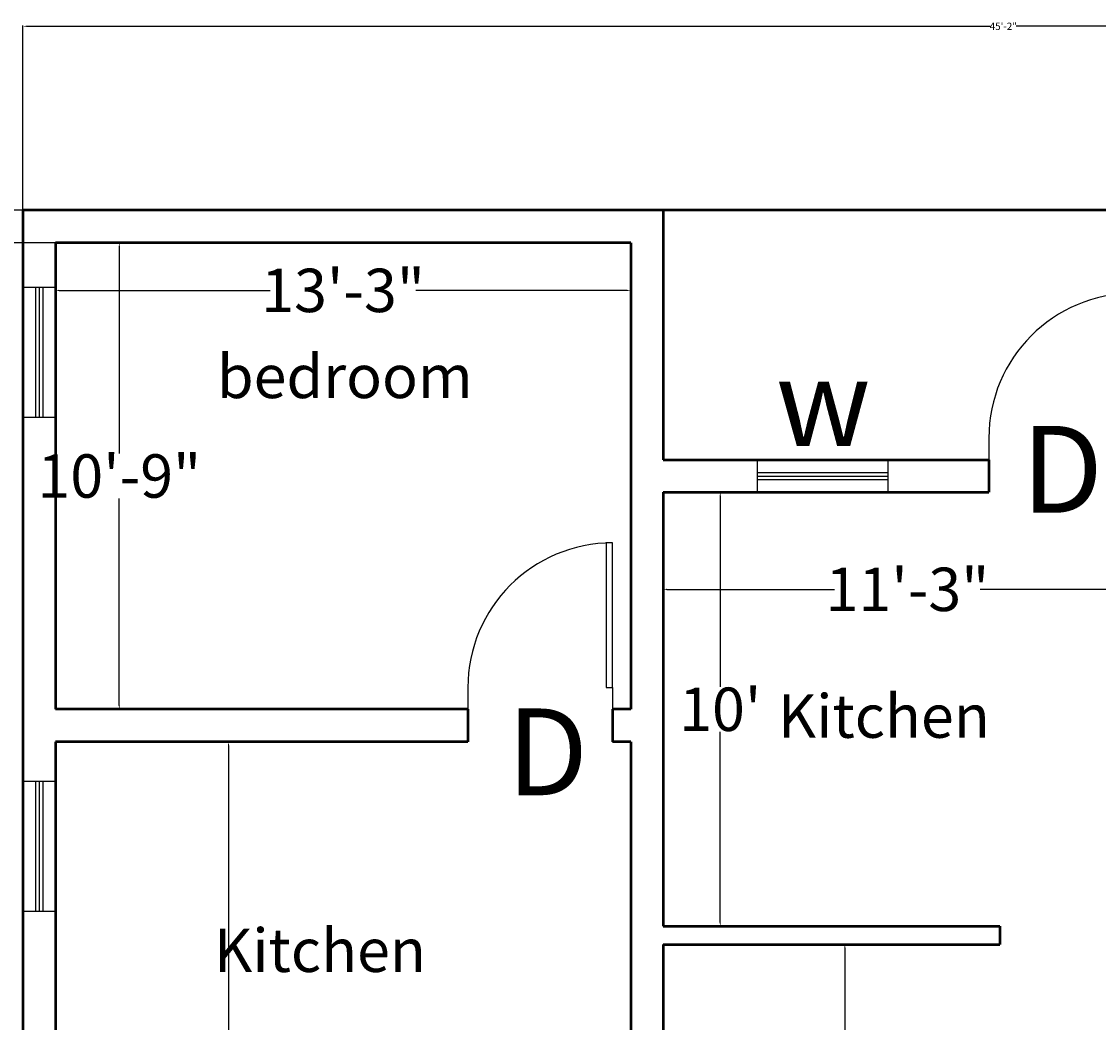
# Model space of a CAD drawing. Units: inches. Extents: x 409 to 7572, y 7 to 725.
# Tile 24 of 38: x 4326 to 4623, y 448 to 725. Entities that reach past the tile are written whole.
import ezdxf

# ---------------------------------------------------------------- set-up
doc = ezdxf.new("R2010")
doc.units = ezdxf.units.IN
doc.header["$MEASUREMENT"] = 0
for name, color, linetype, lineweight in [('A-ANNO-DIMS', 2, 'Continuous', 18), ('A-ANNO-SYMB', 3, 'Continuous', 25), ('A-AREA-IDEN', 7, 'Continuous', 25), ('A-DOOR', 3, 'Continuous', 25), ('A-GLAZ', 4, 'Continuous', 25), ('A-WALL', 7, 'Continuous', 50)]:
    doc.layers.add(name, color=color, linetype=linetype, lineweight=lineweight)
doc.styles.get("Standard").update_dxf_attribs({"font": 'arial.ttf'})
doc.dimstyles.get("Standard").update_dxf_attribs({"dimtxt": 2, "dimasz": 1, "dimexe": 0.18, "dimexo": 0.0625, "dimgap": 0.09, "dimtad": 0, "dimtih": 1, "dimtoh": 1, "dimdec": 0, "dimzin": 0, "dimdsep": 46, "dimlunit": 3, "dimtxsty": 'Standard', "dimcen": 0.09, "dimadec": 0, "dimazin": 0, "dimtfac": 1, "dimtdec": 0, "dimtofl": 0, "dimtmove": 0, "dimatfit": 3, "dimfxl": 1, "dimtolj": 1, "dimtzin": 0, "dimarcsym": 0})

# ---------------------------------------------------------------- blocks, each defined once
blk = doc.blocks.new('*U2')
for p, q in [((0, 0), (0, -6)), ((-40, 0), (-40, -6))]:
    blk.add_line(p, q)
blk.add_lwpolyline([(0, 0), (0, 40), (-1.75, 40), (-1.75, 0)], close=True)
blk.add_arc((0, 0), 40, 90, 180)
blk = doc.blocks.new('*D99')
at = {"layer": 'A-ANNO-DIMS', "color": 0, "lineweight": -2, "transparency": 16777216}
for p, q in [((4335, 663.53), (4352.77, 663.53)), ((4352.59, 662.53), (4352.59, 605.25)), ((4352.59, 535.53), (4352.59, 592.81)), ((4335, 534.53), (4352.77, 534.53))]:
    blk.add_line(p, q, dxfattribs=at)
at = {"layer": 'A-ANNO-DIMS', "color": 0, "transparency": 16777216}
for points in [[(4352.43, 662.53), (4352.76, 662.53), (4352.59, 663.53)], [(4352.43, 535.53), (4352.76, 535.53), (4352.59, 534.53)]]:
    blk.add_solid(points, dxfattribs=at)
at = {"layer": 'DEFPOINTS', "color": 0, "transparency": 16777216}
for p in [(4334.94, 663.53), (4334.94, 534.53), (4352.59, 534.53)]:
    blk.add_point(p, dxfattribs=at)
at = {"layer": 'A-ANNO-DIMS', "color": 0, "transparency": 16777216, "insert": (4352.59, 599.03), "char_height": 2, "attachment_point": 5}
blk.add_mtext('\\A1;{\\H6x;10\'-9"}', dxfattribs=at)
blk = doc.blocks.new('*D100')
at = {"layer": 'A-ANNO-DIMS', "color": 0, "lineweight": -2, "transparency": 16777216}
for p, q in [((4334.94, 663.47), (4334.94, 650.17)), ((4493.94, 663.47), (4493.94, 650.17)), ((4335.94, 650.35), (4394.3, 650.35)), ((4492.94, 650.35), (4434.58, 650.35))]:
    blk.add_line(p, q, dxfattribs=at)
at = {"layer": 'A-ANNO-DIMS', "color": 0, "transparency": 16777216}
for points in [[(4335.94, 650.52), (4335.94, 650.19), (4334.94, 650.35)], [(4492.94, 650.52), (4492.94, 650.19), (4493.94, 650.35)]]:
    blk.add_solid(points, dxfattribs=at)
at = {"layer": 'DEFPOINTS', "color": 0, "transparency": 16777216}
for p in [(4334.94, 663.53), (4493.94, 663.53), (4493.94, 650.35)]:
    blk.add_point(p, dxfattribs=at)
at = {"layer": 'A-ANNO-DIMS', "color": 0, "transparency": 16777216, "insert": (4414.44, 650.35), "char_height": 2, "attachment_point": 5}
blk.add_mtext('\\A1;{\\H6x;13\'-3"}', dxfattribs=at)
blk = doc.blocks.new('*D109')
at = {"layer": 'A-ANNO-DIMS', "color": 0, "lineweight": -2, "transparency": 16777216}
for p, q in [((4503, 594.53), (4518.88, 594.53)), ((4518.7, 593.53), (4518.7, 540.75)), ((4518.7, 475.53), (4518.7, 528.31)), ((4503, 474.53), (4518.88, 474.53))]:
    blk.add_line(p, q, dxfattribs=at)
at = {"layer": 'A-ANNO-DIMS', "color": 0, "transparency": 16777216}
for points in [[(4518.53, 593.53), (4518.86, 593.53), (4518.7, 594.53)], [(4518.53, 475.53), (4518.86, 475.53), (4518.7, 474.53)]]:
    blk.add_solid(points, dxfattribs=at)
at = {"layer": 'DEFPOINTS', "color": 0, "transparency": 16777216}
for p in [(4502.94, 594.53), (4502.94, 474.53), (4518.7, 474.53)]:
    blk.add_point(p, dxfattribs=at)
at = {"layer": 'A-ANNO-DIMS', "color": 0, "transparency": 16777216, "insert": (4518.7, 534.53), "char_height": 2, "attachment_point": 5}
blk.add_mtext("\\A1;{\\H6x;10'}", dxfattribs=at)
blk = doc.blocks.new('*D111')
at = {"layer": 'A-ANNO-DIMS', "color": 0, "lineweight": -2, "transparency": 16777216}
for p, q in [((4391.88, 525.53), (4382.6, 525.53)), ((4382.78, 524.53), (4382.78, 428.65)), ((4382.78, 320.53), (4382.78, 416.42)), ((4399.88, 319.53), (4382.6, 319.53))]:
    blk.add_line(p, q, dxfattribs=at)
at = {"layer": 'A-ANNO-DIMS', "color": 0, "transparency": 16777216}
for points in [[(4382.61, 524.53), (4382.94, 524.53), (4382.78, 525.53)], [(4382.61, 320.53), (4382.94, 320.53), (4382.78, 319.53)]]:
    blk.add_solid(points, dxfattribs=at)
at = {"layer": 'DEFPOINTS', "color": 0, "transparency": 16777216}
for p in [(4391.94, 525.53), (4382.78, 319.53), (4399.94, 319.53)]:
    blk.add_point(p, dxfattribs=at)
at = {"layer": 'A-ANNO-DIMS', "color": 0, "transparency": 16777216, "insert": (4382.78, 422.53), "char_height": 2, "attachment_point": 5}
blk.add_mtext('\\A1;{\\H6x;17\'-2"}', dxfattribs=at)
blk = doc.blocks.new('*D107')
at = {"layer": 'A-ANNO-DIMS', "color": 0, "lineweight": -2, "transparency": 16777216}
for p, q in [((4502.94, 563.4), (4502.94, 567.87)), ((4503.94, 567.69), (4550.3, 567.69)), ((4636.94, 567.69), (4590.58, 567.69)), ((4637.94, 563.4), (4637.94, 567.87))]:
    blk.add_line(p, q, dxfattribs=at)
at = {"layer": 'A-ANNO-DIMS', "color": 0, "transparency": 16777216}
for points in [[(4503.94, 567.86), (4503.94, 567.52), (4502.94, 567.69)], [(4636.94, 567.86), (4636.94, 567.52), (4637.94, 567.69)]]:
    blk.add_solid(points, dxfattribs=at)
at = {"layer": 'DEFPOINTS', "color": 0, "transparency": 16777216}
for p in [(4637.94, 567.69), (4502.94, 563.33), (4637.94, 563.33)]:
    blk.add_point(p, dxfattribs=at)
at = {"layer": 'A-ANNO-DIMS', "color": 0, "transparency": 16777216, "insert": (4570.44, 567.69), "char_height": 2, "attachment_point": 5}
blk.add_mtext('\\A1;{\\H6x;11\'-3"}', dxfattribs=at)
blk = doc.blocks.new('*D112')
at = {"layer": 'A-ANNO-DIMS', "color": 0, "lineweight": -2, "transparency": 16777216}
for p, q in [((4557.2, 469.53), (4552.96, 469.53)), ((4553.14, 468.53), (4553.14, 409.65)), ((4553.14, 338.53), (4553.14, 397.42)), ((4558.38, 337.53), (4552.96, 337.53))]:
    blk.add_line(p, q, dxfattribs=at)
at = {"layer": 'A-ANNO-DIMS', "color": 0, "transparency": 16777216}
for points in [[(4552.97, 468.53), (4553.31, 468.53), (4553.14, 469.53)], [(4552.97, 338.53), (4553.31, 338.53), (4553.14, 337.53)]]:
    blk.add_solid(points, dxfattribs=at)
at = {"layer": 'DEFPOINTS', "color": 0, "transparency": 16777216}
for p in [(4557.27, 469.53), (4553.14, 337.53), (4558.44, 337.53)]:
    blk.add_point(p, dxfattribs=at)
at = {"layer": 'A-ANNO-DIMS', "color": 0, "transparency": 16777216, "insert": (4553.14, 403.53), "char_height": 2, "attachment_point": 5}
blk.add_mtext("\\A1;{\\H6x;11'}", dxfattribs=at)
blk = doc.blocks.new('*D118')
at = {"layer": 'A-ANNO-DIMS', "color": 0, "lineweight": -2, "transparency": 16777216}
for p, q in [((4325.94, 672.59), (4325.94, 723.56)), ((4326.94, 723.38), (4593.38, 723.38)), ((4866.94, 723.38), (4600.51, 723.38)), ((4867.94, 672.59), (4867.94, 723.56))]:
    blk.add_line(p, q, dxfattribs=at)
at = {"layer": 'A-ANNO-DIMS', "color": 0, "transparency": 16777216}
for points in [[(4326.94, 723.55), (4326.94, 723.22), (4325.94, 723.38)], [(4866.94, 723.55), (4866.94, 723.22), (4867.94, 723.38)]]:
    blk.add_solid(points, dxfattribs=at)
at = {"layer": 'DEFPOINTS', "color": 0, "transparency": 16777216}
for p in [(4325.94, 723.38), (4325.94, 672.53), (4867.94, 672.53)]:
    blk.add_point(p, dxfattribs=at)
at = {"layer": 'A-ANNO-DIMS', "color": 0, "transparency": 16777216, "insert": (4596.94, 723.38), "char_height": 2, "attachment_point": 5}
blk.add_mtext('\\A1;45\'-2"', dxfattribs=at)
blk = doc.blocks.new('*D104')
at = {"layer": 'A-ANNO-DIMS', "color": 0, "lineweight": -2, "transparency": 16777216}
for p, q in [((4325.88, 672.53), (4214.98, 672.53)), ((4215.16, 671.53), (4215.16, 544.65)), ((4215.16, 405.53), (4215.16, 532.42)), ((4325.88, 404.53), (4214.98, 404.53))]:
    blk.add_line(p, q, dxfattribs=at)
at = {"layer": 'A-ANNO-DIMS', "color": 0, "transparency": 16777216}
for points in [[(4214.99, 671.53), (4215.33, 671.53), (4215.16, 672.53)], [(4214.99, 405.53), (4215.33, 405.53), (4215.16, 404.53)]]:
    blk.add_solid(points, dxfattribs=at)
at = {"layer": 'DEFPOINTS', "color": 0, "transparency": 16777216}
for p in [(4325.94, 672.53), (4215.16, 404.53), (4325.94, 404.53)]:
    blk.add_point(p, dxfattribs=at)
at = {"layer": 'A-ANNO-DIMS', "color": 0, "transparency": 16777216, "insert": (4215.16, 538.53), "char_height": 2, "attachment_point": 5}
blk.add_mtext('\\A1;{\\H6x;22\'-4"}', dxfattribs=at)
blk = doc.blocks.new('*D93')
at = {"layer": 'A-ANNO-DIMS', "color": 0, "lineweight": -2, "transparency": 16777216}
for p, q in [((4325.88, 672.53), (4161.52, 672.53)), ((4161.7, 671.53), (4161.7, 420.75)), ((4161.7, 157.53), (4161.7, 408.31)), ((4325.88, 156.53), (4161.52, 156.53))]:
    blk.add_line(p, q, dxfattribs=at)
at = {"layer": 'A-ANNO-DIMS', "color": 0, "transparency": 16777216}
for points in [[(4161.54, 671.53), (4161.87, 671.53), (4161.7, 672.53)], [(4161.54, 157.53), (4161.87, 157.53), (4161.7, 156.53)]]:
    blk.add_solid(points, dxfattribs=at)
at = {"layer": 'DEFPOINTS', "color": 0, "transparency": 16777216}
for p in [(4325.94, 672.53), (4161.7, 156.53), (4325.94, 156.53)]:
    blk.add_point(p, dxfattribs=at)
at = {"layer": 'A-ANNO-DIMS', "color": 0, "transparency": 16777216, "insert": (4161.7, 414.53), "char_height": 2, "attachment_point": 5}
blk.add_mtext("\\A1;{\\H6x;43'}", dxfattribs=at)
blk = doc.blocks.new('WIN-36')
for p, q in [((1699.82, 514.65), (1699.82, 478.65)), ((1700.82, 514.65), (1700.82, 478.65)), ((1701.82, 514.65), (1701.82, 478.65))]:
    blk.add_line(p, q)
blk.add_lwpolyline([(1705.32, 514.65), (1705.32, 478.65), (1696.32, 478.65), (1696.32, 514.65)], close=True)
blk = doc.blocks.new('*D188')
at = {"layer": 'A-ANNO-DIMS', "color": 0, "lineweight": -2, "transparency": 16777216}
for p, q in [((4325.88, 672.53), (4239.26, 672.53)), ((4239.44, 671.53), (4239.44, 669.14)), ((4239.44, 664.53), (4239.44, 666.92)), ((4334.88, 663.53), (4239.26, 663.53))]:
    blk.add_line(p, q, dxfattribs=at)
at = {"layer": 'A-ANNO-DIMS', "color": 0, "transparency": 16777216}
for points in [[(4239.27, 671.53), (4239.61, 671.53), (4239.44, 672.53)], [(4239.27, 664.53), (4239.61, 664.53), (4239.44, 663.53)]]:
    blk.add_solid(points, dxfattribs=at)
at = {"layer": 'DEFPOINTS', "color": 0, "transparency": 16777216}
for p in [(4325.94, 672.53), (4239.44, 663.53), (4334.94, 663.53)]:
    blk.add_point(p, dxfattribs=at)
at = {"layer": 'A-ANNO-DIMS', "color": 0, "transparency": 16777216, "insert": (4239.44, 668.03), "char_height": 2, "attachment_point": 5}
blk.add_mtext('\\A1;0\'-9"', dxfattribs=at)

msp = doc.modelspace()

# ---------------------------------------------------------------- linework, layer by layer
at = {"layer": 'A-WALL'}
for p, q in [((4867.94, 672.53), (4325.94, 672.53)), ((4325.94, 672.53), (4325.94, 404.53)), ((4502.94, 672.53), (4502.94, 603.53)), ((4493.94, 663.53), (4334.94, 663.53)), ((4334.94, 663.53), (4334.94, 534.53)), ((4493.94, 663.53), (4493.94, 534.53)), ((4493.94, 663.53), (4493.94, 534.53)), ((4502.94, 603.53), (4592.94, 603.53)), ((4592.94, 603.53), (4592.94, 594.53)), ((4502.94, 594.53), (4592.94, 594.53)), ((4502.94, 594.53), (4502.94, 474.53)), ((4448.94, 534.53), (4334.94, 534.53)), ((4448.94, 534.53), (4448.94, 525.53)), ((4493.94, 534.53), (4488.94, 534.53)), ((4488.94, 534.53), (4488.94, 525.53)), ((4448.94, 525.53), (4334.94, 525.53)), ((4334.94, 525.53), (4334.94, 404.53)), ((4493.94, 525.53), (4488.94, 525.53)), ((4493.94, 525.53), (4493.94, 319.53)), ((4502.94, 474.53), (4595.94, 474.53)), ((4595.94, 474.53), (4595.94, 469.53)), ((4502.94, 469.53), (4595.94, 469.53)), ((4502.94, 469.53), (4502.94, 337.53))]:
    msp.add_line(p, q, dxfattribs=at)

# ---------------------------------------------------------------- block references
at = {"layer": 'A-DOOR'}
for p in [(4632.94, 609.53), (4488.94, 540.53)]:
    msp.add_blockref('*U2', p, dxfattribs=at)
at = {"layer": 'A-GLAZ'}
for p in [(2629.62, 136.58), (2629.62, 0)]:
    msp.add_blockref('WIN-36', p, dxfattribs=at)
at = {"layer": 'A-GLAZ', "rotation": 89.99999999999812}
msp.add_blockref('WIN-36', (5043.68, -1101.79), dxfattribs=at)

# ---------------------------------------------------------------- texts
at = {"layer": 'A-ANNO-SYMB', "char_height": 24, "attachment_point": 1}
for s, width, insert in [('w', 18.2582, (4534.03, 631.37)), ('D', 19.1972, (4601.97, 612.87)), ('D', 19.1972, (4459.66, 534.75))]:
    msp.add_mtext_dynamic_manual_height_columns(s, width=width, gutter_width=1, heights=[0], dxfattribs=dict(at, insert=insert))
at = {"layer": 'A-AREA-IDEN', "char_height": 12, "attachment_point": 1}
for s, width, insert in [('bedroom', 40.9017, (4379.6, 632.57)), ('Kitchen ', 61.5504, (4534.63, 538.64)), ('Kitchen ', 61.5504, (4378.77, 473.89))]:
    msp.add_mtext_dynamic_manual_height_columns(s, width=width, gutter_width=1, heights=[0], dxfattribs=dict(at, insert=insert))

# ---------------------------------------------------------------- dimensions: what is measured, and where the dimension line sits
at = {"layer": 'A-ANNO-DIMS'}
dim = msp.add_linear_dim(base=(4325.94, 723.38), p1=(4867.94, 672.53), p2=(4325.94, 672.53), dimstyle='Standard', override={"dimclrd": 0, "dimclre": 0, "dimclrt": 0}, dxfattribs=at)
dim.commit()
dim.dimension.update_dxf_attribs({"geometry": '*D118', "text_midpoint": (4596.94, 723.38)})
for base, p1, p2, picture, middle in [((4161.7, 156.53), (4325.94, 672.53), (4325.94, 156.53), '*D93', (4161.7, 414.53)), ((4215.16, 404.53), (4325.94, 672.53), (4325.94, 404.53), '*D104', (4215.16, 538.53)), ((4352.59, 534.53), (4334.94, 663.53), (4334.94, 534.53), '*D99', (4352.59, 599.03)), ((4518.7, 474.53), (4502.94, 594.53), (4502.94, 474.53), '*D109', (4518.7, 534.53)), ((4553.14, 337.53), (4557.27, 469.53), (4558.44, 337.53), '*D112', (4553.14, 403.53))]:
    dim = msp.add_linear_dim(base=base, p1=p1, p2=p2, angle=90, text='{\\H6x;<>}', dimstyle='Standard', override={"dimclrd": 0, "dimclre": 0, "dimclrt": 0}, dxfattribs=at)
    dim.commit()
    dim.dimension.update_dxf_attribs({"geometry": picture, "text_midpoint": middle})
dim = msp.add_linear_dim(base=(4239.44, 663.53), p1=(4325.94, 672.53), p2=(4334.94, 663.53), angle=90, dimstyle='Standard', override={"dimdec": 1, "dimlfac": 1, "dimrnd": 0, "dimzin": 1, "dimdsep": 46, "dimlunit": 4, "dimfrac": 2}, dxfattribs=at)
dim.commit()
dim.dimension.update_dxf_attribs({"geometry": '*D188', "text_midpoint": (4239.44, 668.03)})
for base, p1, p2, picture, middle in [((4493.94, 650.35), (4334.94, 663.53), (4493.94, 663.53), '*D100', (4414.44, 650.35)), ((4637.94, 567.69), (4502.94, 563.33), (4637.94, 563.33), '*D107', (4570.44, 567.69))]:
    dim = msp.add_linear_dim(base=base, p1=p1, p2=p2, text='{\\H6x;<>}', dimstyle='Standard', override={"dimclrd": 0, "dimclre": 0, "dimclrt": 0}, dxfattribs=at)
    dim.commit()
    dim.dimension.update_dxf_attribs({"geometry": picture, "text_midpoint": middle})
dim = msp.add_linear_dim(base=(4382.78, 319.53), p1=(4391.94, 525.53), p2=(4399.94, 319.53), angle=90, text='{\\H6x;<>}', dimstyle='Standard', override={"dimclrd": 0, "dimclre": 0, "dimclrt": 0}, dxfattribs=at)
dim.commit()
dim.dimension.update_dxf_attribs({"geometry": '*D111', "text_midpoint": (4382.78, 422.53), "dimtype": 160})

doc.saveas('drawing.dxf')
